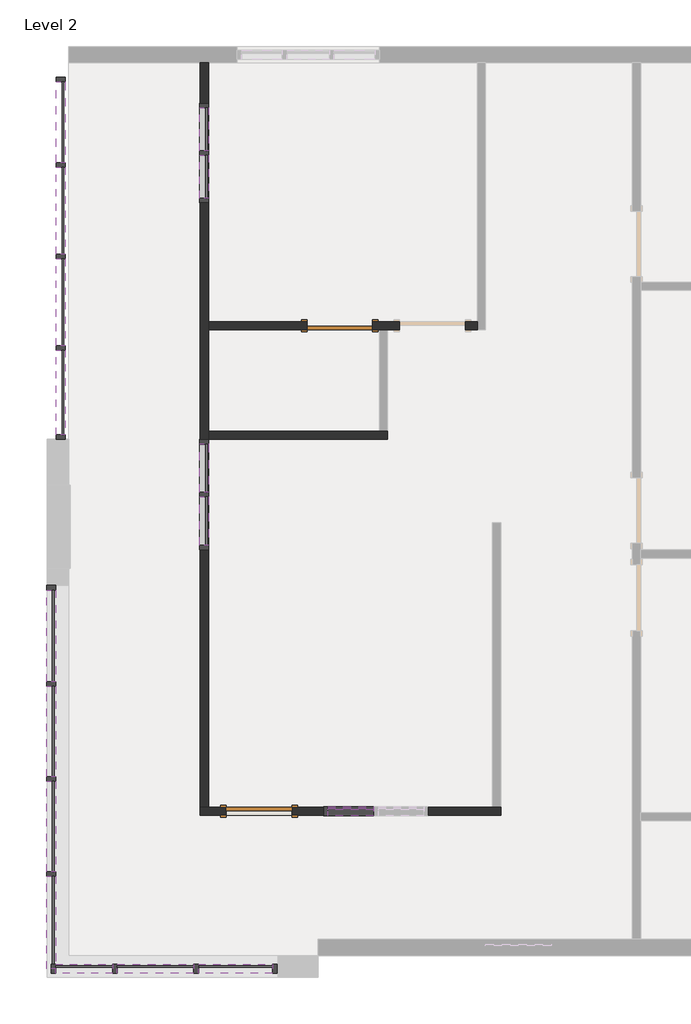
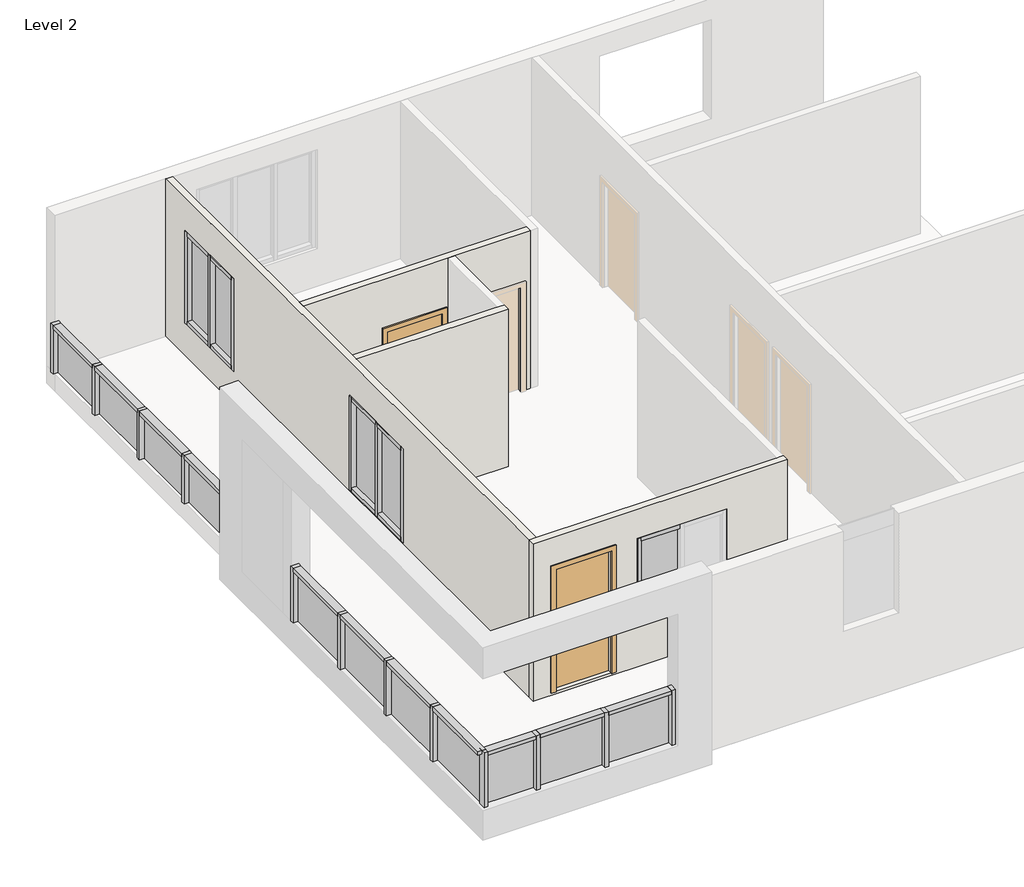
# One storey, part 1 of 2: 41 members, 16 plates, 4 walls, 2 doors.
"""IFC4 building model written with IfcOpenShell, lengths in millimetres."""

from ifc_helpers import new_model, si_unit, origin, place, context, project, spatial, faceted_brep, transform, mapped, element, save
from components import door_305aa2a5, member_a400357f, member_bc7c5251, member_6d802792, member_051277f3, member_fa50fb7e, member_1e79e512, member_04adda39, member_6ffa5180, member_e6b9f524, member_19f58c97, member_63803c1e, member_77473497, member_3cc93373, member_e1cb8a7d, member_bcb6a316, member_cba00588, member_798c2a08, member_45f34f4c, member_e49f56fc, member_c4de40ee, member_13dc6413, member_6ef8dc49, member_eb96f34d, system_panel_glazed_b36345c5, system_panel_glazed_219b4c74, system_panel_glazed_d508df5b, system_panel_glazed_98635403, system_panel_glazed_7a6fc0cf, system_panel_glazed_66c18ae2, system_panel_glazed_0daebeb7, system_panel_glazed_36a05233, system_panel_glazed_4373b602, system_panel_glazed_38c9bce4, system_panel_glazed_4a7c210e, system_panel_glazed_37b2116f

model = new_model("IFC4")

# Units and contexts
model_context = context("Model", 3, world=origin())
ifc_project = project(units=[si_unit("LENGTHUNIT", "METRE", prefix="MILLI")], contexts=[model_context])

# Site, building, storey
site = spatial("IfcSite", under=ifc_project)
building = spatial("IfcBuilding", under=site)
storey = spatial("IfcBuildingStorey", under=building, Name="Level 2", Elevation=3048.0)

# Doors
placement = place(None, origin())
door_shape = door_305aa2a5(model_context)
element("IfcDoor", 1, ObjectType="Single-Flush : 36\" x 84\"", at=placement, inside=storey, context=model_context, shape_type="MappedRepresentation", body=[
    mapped(door_shape, transform((-16492.8503587, -5110.3526331, 3048.0), x_axis=(1.0, 0.0, 0.0), y_axis=(0.0, 1.0, 0.0), z_axis=(0.0, 0.0, 1.0))),
])
element("IfcDoor", 2, ObjectType="Single-Flush : 36\" x 84\"", at=placement, inside=storey, context=model_context, shape_type="MappedRepresentation", body=[
    mapped(door_shape, transform((-17616.8003587, -11866.7526331, 3403.6), x_axis=(-1.0, 0.0, 0.0), y_axis=(0.0, -1.0, 0.0), z_axis=(0.0, 0.0, 1.0))),
])

# Members
member_shape = member_a400357f(model_context)
element("IfcMember", 3, ObjectType="Rectangular Mullion : 2.5\" x 5\" rectangular", at=placement, inside=storey, context=model_context, shape_type="MappedRepresentation", body=[
    mapped(member_shape, transform((-18378.8003587, -2671.9526331, 5536.2113847), x_axis=(0.0, 0.0, 1.0), y_axis=(-1.0, 0.0, 0.0), z_axis=(0.0, -1.0, 0.0))),
])
element("IfcMember", 4, ObjectType="Rectangular Mullion : 2.5\" x 5\" rectangular", at=placement, inside=storey, context=model_context, shape_type="MappedRepresentation", body=[
    mapped(member_shape, transform((-18378.8003587, -3332.3526331, 5536.2113847), x_axis=(0.0, 0.0, 1.0), y_axis=(-1.0, 0.0, 0.0), z_axis=(0.0, -1.0, 0.0))),
])
member_2_shape = member_bc7c5251(model_context)
element("IfcMember", 5, ObjectType="Rectangular Mullion : 2.5\" x 5\" rectangular", at=placement, inside=storey, context=model_context, shape_type="MappedRepresentation", body=[
    mapped(member_2_shape, transform((-18378.8003587, -2703.7026331, 3927.5904931), x_axis=(0.0, -1.0, 0.0), y_axis=(-1.0, 0.0, 0.0), z_axis=(0.0, 0.0, -1.0))),
])
element("IfcMember", 6, ObjectType="Rectangular Mullion : 2.5\" x 5\" rectangular", at=placement, inside=storey, context=model_context, shape_type="MappedRepresentation", body=[
    mapped(member_shape, transform((-18378.8003587, -2735.4526331, 3927.5904931), x_axis=(0.0, 0.0, -1.0), y_axis=(-1.0, 0.0, 0.0), z_axis=(0.0, 1.0, 0.0))),
])
element("IfcMember", 7, ObjectType="Rectangular Mullion : 2.5\" x 5\" rectangular", at=placement, inside=storey, context=model_context, shape_type="MappedRepresentation", body=[
    mapped(member_shape, transform((-18378.8003587, -2075.0526331, 3927.5904931), x_axis=(0.0, 0.0, -1.0), y_axis=(-1.0, 0.0, 0.0), z_axis=(0.0, 1.0, 0.0))),
])
member_3_shape = member_6d802792(model_context)
element("IfcMember", 8, ObjectType="Rectangular Mullion : 2.5\" x 5\" rectangular", at=placement, inside=storey, context=model_context, shape_type="MappedRepresentation", body=[
    mapped(member_3_shape, transform((-18378.8003587, -3395.8526331, 3927.5904931), x_axis=(0.0, -1.0, 0.0), y_axis=(-1.0, 0.0, 0.0), z_axis=(0.0, 0.0, -1.0))),
])
element("IfcMember", 9, ObjectType="Rectangular Mullion : 2.5\" x 5\" rectangular", at=placement, inside=storey, context=model_context, shape_type="MappedRepresentation", body=[
    mapped(member_3_shape, transform((-18378.8003587, -2011.5526331, 5536.2113847), x_axis=(0.0, 1.0, 0.0), y_axis=(-1.0, 0.0, 0.0), z_axis=(0.0, 0.0, 1.0))),
])
member_4_shape = member_051277f3(model_context)
element("IfcMember", 10, ObjectType="Rectangular Mullion : 2.5\" x 5\" rectangular", at=placement, inside=storey, context=model_context, shape_type="MappedRepresentation", body=[
    mapped(member_4_shape, transform((-18378.8003587, -7428.1026331, 5506.8936219), x_axis=(0.0, 0.0, 1.0), y_axis=(-1.0, 0.0, 0.0), z_axis=(0.0, -1.0, 0.0))),
])
element("IfcMember", 11, ObjectType="Rectangular Mullion : 2.5\" x 5\" rectangular", at=placement, inside=storey, context=model_context, shape_type="MappedRepresentation", body=[
    mapped(member_4_shape, transform((-18378.8003587, -8164.7026331, 5506.8936219), x_axis=(0.0, 0.0, 1.0), y_axis=(-1.0, 0.0, 0.0), z_axis=(0.0, -1.0, 0.0))),
])
member_5_shape = member_fa50fb7e(model_context)
element("IfcMember", 12, ObjectType="Rectangular Mullion : 2.5\" x 5\" rectangular", at=placement, inside=storey, context=model_context, shape_type="MappedRepresentation", body=[
    mapped(member_5_shape, transform((-18378.8003587, -7459.8526331, 3873.1435835), x_axis=(0.0, -1.0, 0.0), y_axis=(-1.0, 0.0, 0.0), z_axis=(0.0, 0.0, -1.0))),
])
element("IfcMember", 13, ObjectType="Rectangular Mullion : 2.5\" x 5\" rectangular", at=placement, inside=storey, context=model_context, shape_type="MappedRepresentation", body=[
    mapped(member_4_shape, transform((-18378.8003587, -7491.6026331, 3873.1435835), x_axis=(0.0, 0.0, -1.0), y_axis=(-1.0, 0.0, 0.0), z_axis=(0.0, 1.0, 0.0))),
])
element("IfcMember", 14, ObjectType="Rectangular Mullion : 2.5\" x 5\" rectangular", at=placement, inside=storey, context=model_context, shape_type="MappedRepresentation", body=[
    mapped(member_4_shape, transform((-18378.8003587, -6755.0026331, 3873.1435835), x_axis=(0.0, 0.0, -1.0), y_axis=(-1.0, 0.0, 0.0), z_axis=(0.0, 1.0, 0.0))),
])
member_6_shape = member_1e79e512(model_context)
element("IfcMember", 15, ObjectType="Rectangular Mullion : 2.5\" x 5\" rectangular", at=placement, inside=storey, context=model_context, shape_type="MappedRepresentation", body=[
    mapped(member_6_shape, transform((-18378.8003587, -6691.5026331, 5506.8936219), x_axis=(0.0, 1.0, 0.0), y_axis=(-1.0, 0.0, 0.0), z_axis=(0.0, 0.0, 1.0))),
])
element("IfcMember", 16, ObjectType="Rectangular Mullion : 2.5\" x 5\" rectangular", at=placement, inside=storey, context=model_context, shape_type="MappedRepresentation", body=[
    mapped(member_6_shape, transform((-18378.8003587, -8228.2026331, 3873.1435835), x_axis=(0.0, -1.0, 0.0), y_axis=(-1.0, 0.0, 0.0), z_axis=(0.0, 0.0, -1.0))),
])
member_7_shape = member_04adda39(model_context)
element("IfcMember", 17, ObjectType="Rectangular Mullion : 2.5\" x 5\" rectangular", at=placement, inside=storey, context=model_context, shape_type="MappedRepresentation", body=[
    mapped(member_7_shape, transform((-16019.7753587, -11866.7526331, 5586.8732654), x_axis=(0.0, 0.0, 1.0), y_axis=(0.0, -1.0, 0.0), z_axis=(1.0, 0.0, 0.0))),
])
element("IfcMember", 18, ObjectType="Rectangular Mullion : 2.5\" x 5\" rectangular", at=placement, inside=storey, context=model_context, shape_type="MappedRepresentation", body=[
    mapped(member_7_shape, transform((-16657.9503587, -11866.7526331, 4227.0998045), x_axis=(0.0, 0.0, -1.0), y_axis=(0.0, -1.0, 0.0), z_axis=(-1.0, 0.0, 0.0))),
])
member_8_shape = member_6ffa5180(model_context)
element("IfcMember", 19, ObjectType="Rectangular Mullion : 2.5\" x 5\" rectangular", at=placement, inside=storey, context=model_context, shape_type="MappedRepresentation", body=[
    mapped(member_8_shape, transform((-16721.4503587, -11866.7526331, 5586.8732654), x_axis=(-1.0, 0.0, 0.0), y_axis=(0.0, -1.0, 0.0), z_axis=(0.0, 0.0, 1.0))),
])
member_9_shape = member_e6b9f524(model_context)
element("IfcMember", 20, ObjectType="Rectangular Mullion : 2.5\" x 5\" rectangular", at=placement, inside=storey, context=model_context, shape_type="MappedRepresentation", body=[
    mapped(member_9_shape, transform((-20379.0503587, -2841.0830211, 4408.9968859), x_axis=(0.0, 0.0, 1.0), y_axis=(-1.0, 0.0, 0.0), z_axis=(0.0, -1.0, 0.0))),
])
member_10_shape = member_19f58c97(model_context)
element("IfcMember", 21, ObjectType="Rectangular Mullion : 2.5\" x 5\" rectangular", at=placement, inside=storey, context=model_context, shape_type="MappedRepresentation", body=[
    mapped(member_10_shape, transform((-20379.0503587, -1653.6330211, 4408.9968859), x_axis=(0.0, 1.0, 0.0), y_axis=(-1.0, 0.0, 0.0), z_axis=(0.0, 0.0, 1.0))),
])
member_11_shape = member_63803c1e(model_context)
element("IfcMember", 22, ObjectType="Rectangular Mullion : 2.5\" x 5\" rectangular", at=placement, inside=storey, context=model_context, shape_type="MappedRepresentation", body=[
    mapped(member_11_shape, transform((-20379.0503587, -2872.8330211, 3560.986402), x_axis=(0.0, -1.0, 0.0), y_axis=(-1.0, 0.0, 0.0), z_axis=(0.0, 0.0, -1.0))),
])
element("IfcMember", 23, ObjectType="Rectangular Mullion : 2.5\" x 5\" rectangular", at=placement, inside=storey, context=model_context, shape_type="MappedRepresentation", body=[
    mapped(member_11_shape, transform((-20379.0503587, -4145.7228918, 3560.986402), x_axis=(0.0, -1.0, 0.0), y_axis=(-1.0, 0.0, 0.0), z_axis=(0.0, 0.0, -1.0))),
])
element("IfcMember", 24, ObjectType="Rectangular Mullion : 2.5\" x 5\" rectangular", at=placement, inside=storey, context=model_context, shape_type="MappedRepresentation", body=[
    mapped(member_11_shape, transform((-20379.0503587, -5418.6127624, 3560.986402), x_axis=(0.0, -1.0, 0.0), y_axis=(-1.0, 0.0, 0.0), z_axis=(0.0, 0.0, -1.0))),
])
member_12_shape = member_77473497(model_context)
element("IfcMember", 25, ObjectType="Rectangular Mullion : 2.5\" x 5\" rectangular", at=placement, inside=storey, context=model_context, shape_type="MappedRepresentation", body=[
    mapped(member_12_shape, transform((-20379.0503587, -5386.8627624, 4408.9968859), x_axis=(0.0, 0.0, 1.0), y_axis=(-1.0, 0.0, 0.0), z_axis=(0.0, -1.0, 0.0))),
])
element("IfcMember", 26, ObjectType="Rectangular Mullion : 2.5\" x 5\" rectangular", at=placement, inside=storey, context=model_context, shape_type="MappedRepresentation", body=[
    mapped(member_12_shape, transform((-20379.0503587, -4113.9728918, 4408.9968859), x_axis=(0.0, 0.0, 1.0), y_axis=(-1.0, 0.0, 0.0), z_axis=(0.0, -1.0, 0.0))),
])
member_13_shape = member_3cc93373(model_context)
element("IfcMember", 27, ObjectType="Rectangular Mullion : 2.5\" x 5\" rectangular", at=placement, inside=storey, context=model_context, shape_type="MappedRepresentation", body=[
    mapped(member_13_shape, transform((-20379.0503587, -6628.0026331, 4408.9968859), x_axis=(0.0, 0.0, 1.0), y_axis=(-1.0, 0.0, 0.0), z_axis=(0.0, -1.0, 0.0))),
])
element("IfcMember", 28, ObjectType="Rectangular Mullion : 2.5\" x 5\" rectangular", at=placement, inside=storey, context=model_context, shape_type="MappedRepresentation", body=[
    mapped(member_10_shape, transform((-20379.0503587, -6691.5026331, 3560.986402), x_axis=(0.0, -1.0, 0.0), y_axis=(-1.0, 0.0, 0.0), z_axis=(0.0, 0.0, -1.0))),
])
member_14_shape = member_e1cb8a7d(model_context)
element("IfcMember", 29, ObjectType="Rectangular Mullion : 2.5\" x 5\" rectangular", at=placement, inside=storey, context=model_context, shape_type="MappedRepresentation", body=[
    mapped(member_14_shape, transform((-20512.4003587, -10095.1026331, 3560.986402), x_axis=(0.0, -1.0, 0.0), y_axis=(-1.0, 0.0, 0.0), z_axis=(0.0, 0.0, -1.0))),
])
element("IfcMember", 30, ObjectType="Rectangular Mullion : 2.5\" x 5\" rectangular", at=placement, inside=storey, context=model_context, shape_type="MappedRepresentation", body=[
    mapped(member_14_shape, transform((-20512.4003587, -11415.9026331, 3560.986402), x_axis=(0.0, -1.0, 0.0), y_axis=(-1.0, 0.0, 0.0), z_axis=(0.0, 0.0, -1.0))),
])
element("IfcMember", 31, ObjectType="Rectangular Mullion : 2.5\" x 5\" rectangular", at=placement, inside=storey, context=model_context, shape_type="MappedRepresentation", body=[
    mapped(member_14_shape, transform((-20512.4003587, -12736.7026331, 3560.986402), x_axis=(0.0, -1.0, 0.0), y_axis=(-1.0, 0.0, 0.0), z_axis=(0.0, 0.0, -1.0))),
])
member_15_shape = member_bcb6a316(model_context)
element("IfcMember", 32, ObjectType="Rectangular Mullion : 2.5\" x 5\" rectangular", at=placement, inside=storey, context=model_context, shape_type="MappedRepresentation", body=[
    mapped(member_15_shape, transform((-20512.4003587, -12704.9526331, 4515.4150439), x_axis=(0.0, 0.0, 1.0), y_axis=(-1.0, 0.0, 0.0), z_axis=(0.0, -1.0, 0.0))),
])
element("IfcMember", 33, ObjectType="Rectangular Mullion : 2.5\" x 5\" rectangular", at=placement, inside=storey, context=model_context, shape_type="MappedRepresentation", body=[
    mapped(member_15_shape, transform((-20512.4003587, -11384.1526331, 4515.4150439), x_axis=(0.0, 0.0, 1.0), y_axis=(-1.0, 0.0, 0.0), z_axis=(0.0, -1.0, 0.0))),
])
member_16_shape = member_cba00588(model_context)
element("IfcMember", 34, ObjectType="Rectangular Mullion : 2.5\" x 5\" rectangular", at=placement, inside=storey, context=model_context, shape_type="MappedRepresentation", body=[
    mapped(member_16_shape, transform((-20512.4003587, -10063.3526331, 4515.4150439), x_axis=(0.0, 0.0, 1.0), y_axis=(-1.0, 0.0, 0.0), z_axis=(0.0, -1.0, 0.0))),
])
member_17_shape = member_798c2a08(model_context)
element("IfcMember", 35, ObjectType="Rectangular Mullion : 2.5\" x 5\" rectangular", at=placement, inside=storey, context=model_context, shape_type="MappedRepresentation", body=[
    mapped(member_17_shape, transform((-20512.4003587, -14057.5026331, 4515.4150439), x_axis=(0.0, 0.0, 1.0), y_axis=(-1.0, 0.0, 0.0), z_axis=(0.0, -1.0, 0.0))),
])
member_18_shape = member_45f34f4c(model_context)
element("IfcMember", 36, ObjectType="Rectangular Mullion : 2.5\" x 5\" rectangular", at=placement, inside=storey, context=model_context, shape_type="MappedRepresentation", body=[
    mapped(member_18_shape, transform((-20512.4003587, -8723.5026331, 4515.4150439), x_axis=(0.0, 1.0, 0.0), y_axis=(-1.0, 0.0, 0.0), z_axis=(0.0, 0.0, 1.0))),
])
member_19_shape = member_e49f56fc(model_context)
element("IfcMember", 37, ObjectType="Rectangular Mullion : 2.5\" x 5\" rectangular", at=placement, inside=storey, context=model_context, shape_type="MappedRepresentation", body=[
    mapped(member_19_shape, transform((-19623.4003587, -14057.5026331, 3560.986402), x_axis=(1.0, 0.0, 0.0), y_axis=(0.0, -1.0, 0.0), z_axis=(0.0, 0.0, -1.0))),
])
element("IfcMember", 38, ObjectType="Rectangular Mullion : 2.5\" x 5\" rectangular", at=placement, inside=storey, context=model_context, shape_type="MappedRepresentation", body=[
    mapped(member_19_shape, transform((-18493.1003587, -14057.5026331, 3560.986402), x_axis=(1.0, 0.0, 0.0), y_axis=(0.0, -1.0, 0.0), z_axis=(0.0, 0.0, -1.0))),
])
member_20_shape = member_c4de40ee(model_context)
element("IfcMember", 39, ObjectType="Rectangular Mullion : 2.5\" x 5\" rectangular", at=placement, inside=storey, context=model_context, shape_type="MappedRepresentation", body=[
    mapped(member_20_shape, transform((-18524.8503587, -14057.5026331, 4515.0022133), x_axis=(0.0, 0.0, 1.0), y_axis=(0.0, -1.0, 0.0), z_axis=(1.0, 0.0, 0.0))),
])
member_21_shape = member_13dc6413(model_context)
element("IfcMember", 40, ObjectType="Rectangular Mullion : 2.5\" x 5\" rectangular", at=placement, inside=storey, context=model_context, shape_type="MappedRepresentation", body=[
    mapped(member_21_shape, transform((-19655.1503587, -14057.5026331, 4515.0022133), x_axis=(0.0, 0.0, 1.0), y_axis=(0.0, -1.0, 0.0), z_axis=(1.0, 0.0, 0.0))),
])
member_22_shape = member_6ef8dc49(model_context)
element("IfcMember", 41, ObjectType="Rectangular Mullion : 2.5\" x 5\" rectangular", at=placement, inside=storey, context=model_context, shape_type="MappedRepresentation", body=[
    mapped(member_22_shape, transform((-17426.3003587, -14057.5026331, 4515.0022133), x_axis=(0.0, 0.0, 1.0), y_axis=(0.0, -1.0, 0.0), z_axis=(1.0, 0.0, 0.0))),
])
member_23_shape = member_eb96f34d(model_context)
element("IfcMember", 42, ObjectType="Rectangular Mullion : 2.5\" x 5\" rectangular", at=placement, inside=storey, context=model_context, shape_type="MappedRepresentation", body=[
    mapped(member_23_shape, transform((-20512.4003587, -14057.5026331, 4515.0022133), x_axis=(-1.0, 0.0, 0.0), y_axis=(0.0, -1.0, 0.0), z_axis=(0.0, 0.0, 1.0))),
])
element("IfcMember", 43, ObjectType="Rectangular Mullion : 2.5\" x 5\" rectangular", at=placement, inside=storey, context=model_context, shape_type="MappedRepresentation", body=[
    mapped(member_23_shape, transform((-17362.8003587, -14057.5026331, 3560.986402), x_axis=(1.0, 0.0, 0.0), y_axis=(0.0, -1.0, 0.0), z_axis=(0.0, 0.0, -1.0))),
])

# Plates
system_panel_glazed_shape = system_panel_glazed_b36345c5(model_context)
element("IfcPlate", 44, ObjectType="System Panel : Glazed", at=placement, inside=storey, context=model_context, shape_type="MappedRepresentation", body=[
    mapped(system_panel_glazed_shape, transform((-18378.8003587, -2373.5026331, 3991.0904931), x_axis=(0.0, -1.0, 0.0), y_axis=(1.0, 0.0, 0.0), z_axis=(0.0, 0.0, 1.0))),
])
element("IfcPlate", 45, ObjectType="System Panel : Glazed", at=placement, inside=storey, context=model_context, shape_type="MappedRepresentation", body=[
    mapped(system_panel_glazed_shape, transform((-18378.8003587, -3033.9026331, 3991.0904931), x_axis=(0.0, -1.0, 0.0), y_axis=(1.0, 0.0, 0.0), z_axis=(0.0, 0.0, 1.0))),
])
system_panel_glazed_2_shape = system_panel_glazed_219b4c74(model_context)
element("IfcPlate", 46, ObjectType="System Panel : Glazed", at=placement, inside=storey, context=model_context, shape_type="MappedRepresentation", body=[
    mapped(system_panel_glazed_2_shape, transform((-18378.8003587, -7091.5526331, 3936.6435835), x_axis=(0.0, -1.0, 0.0), y_axis=(1.0, 0.0, 0.0), z_axis=(0.0, 0.0, 1.0))),
])
element("IfcPlate", 47, ObjectType="System Panel : Glazed", at=placement, inside=storey, context=model_context, shape_type="MappedRepresentation", body=[
    mapped(system_panel_glazed_2_shape, transform((-18378.8003587, -7828.1526331, 3936.6435835), x_axis=(0.0, -1.0, 0.0), y_axis=(1.0, 0.0, 0.0), z_axis=(0.0, 0.0, 1.0))),
])
system_panel_glazed_3_shape = system_panel_glazed_d508df5b(model_context)
element("IfcPlate", 48, ObjectType="System Panel : Glazed", at=placement, inside=storey, context=model_context, shape_type="MappedRepresentation", body=[
    mapped(system_panel_glazed_3_shape, transform((-16338.8628587, -11866.7526331, 4290.5998045), x_axis=(1.0, 0.0, 0.0), y_axis=(0.0, 1.0, 0.0), z_axis=(0.0, 0.0, 1.0))),
])
system_panel_glazed_4_shape = system_panel_glazed_98635403(model_context)
element("IfcPlate", 49, ObjectType="System Panel : Glazed", at=placement, inside=storey, context=model_context, shape_type="MappedRepresentation", body=[
    mapped(system_panel_glazed_4_shape, transform((-20379.0503587, -2279.1080211, 3560.986402), x_axis=(0.0, -1.0, 0.0), y_axis=(1.0, 0.0, 0.0), z_axis=(0.0, 0.0, 1.0))),
])
system_panel_glazed_5_shape = system_panel_glazed_7a6fc0cf(model_context)
element("IfcPlate", 50, ObjectType="System Panel : Glazed", at=placement, inside=storey, context=model_context, shape_type="MappedRepresentation", body=[
    mapped(system_panel_glazed_5_shape, transform((-20379.0503587, -3509.2779565, 3560.986402), x_axis=(0.0, -1.0, 0.0), y_axis=(1.0, 0.0, 0.0), z_axis=(0.0, 0.0, 1.0))),
])
element("IfcPlate", 51, ObjectType="System Panel : Glazed", at=placement, inside=storey, context=model_context, shape_type="MappedRepresentation", body=[
    mapped(system_panel_glazed_5_shape, transform((-20379.0503587, -4782.1678271, 3560.986402), x_axis=(0.0, -1.0, 0.0), y_axis=(1.0, 0.0, 0.0), z_axis=(0.0, 0.0, 1.0))),
])
system_panel_glazed_6_shape = system_panel_glazed_66c18ae2(model_context)
element("IfcPlate", 52, ObjectType="System Panel : Glazed", at=placement, inside=storey, context=model_context, shape_type="MappedRepresentation", body=[
    mapped(system_panel_glazed_6_shape, transform((-20379.0503587, -6039.1826978, 3560.986402), x_axis=(0.0, -1.0, 0.0), y_axis=(1.0, 0.0, 0.0), z_axis=(0.0, 0.0, 1.0))),
])
system_panel_glazed_7_shape = system_panel_glazed_0daebeb7(model_context)
element("IfcPlate", 53, ObjectType="System Panel : Glazed", at=placement, inside=storey, context=model_context, shape_type="MappedRepresentation", body=[
    mapped(system_panel_glazed_7_shape, transform((-20512.4003587, -9425.1776331, 3560.986402), x_axis=(0.0, -1.0, 0.0), y_axis=(1.0, 0.0, 0.0), z_axis=(0.0, 0.0, 1.0))),
])
system_panel_glazed_8_shape = system_panel_glazed_36a05233(model_context)
element("IfcPlate", 54, ObjectType="System Panel : Glazed", at=placement, inside=storey, context=model_context, shape_type="MappedRepresentation", body=[
    mapped(system_panel_glazed_8_shape, transform((-20512.4003587, -10755.5026331, 3560.986402), x_axis=(0.0, -1.0, 0.0), y_axis=(1.0, 0.0, 0.0), z_axis=(0.0, 0.0, 1.0))),
])
element("IfcPlate", 55, ObjectType="System Panel : Glazed", at=placement, inside=storey, context=model_context, shape_type="MappedRepresentation", body=[
    mapped(system_panel_glazed_8_shape, transform((-20512.4003587, -12076.3026331, 3560.986402), x_axis=(0.0, -1.0, 0.0), y_axis=(1.0, 0.0, 0.0), z_axis=(0.0, 0.0, 1.0))),
])
system_panel_glazed_9_shape = system_panel_glazed_4373b602(model_context)
element("IfcPlate", 56, ObjectType="System Panel : Glazed", at=placement, inside=storey, context=model_context, shape_type="MappedRepresentation", body=[
    mapped(system_panel_glazed_9_shape, transform((-20512.4003587, -13412.9776331, 3560.986402), x_axis=(0.0, -1.0, 0.0), y_axis=(1.0, 0.0, 0.0), z_axis=(0.0, 0.0, 1.0))),
])
system_panel_glazed_10_shape = system_panel_glazed_38c9bce4(model_context)
element("IfcPlate", 57, ObjectType="System Panel : Glazed", at=placement, inside=storey, context=model_context, shape_type="MappedRepresentation", body=[
    mapped(system_panel_glazed_10_shape, transform((-20052.0253587, -14057.5026331, 3560.986402), x_axis=(1.0, 0.0, 0.0), y_axis=(0.0, 1.0, 0.0), z_axis=(0.0, 0.0, 1.0))),
])
system_panel_glazed_11_shape = system_panel_glazed_4a7c210e(model_context)
element("IfcPlate", 58, ObjectType="System Panel : Glazed", at=placement, inside=storey, context=model_context, shape_type="MappedRepresentation", body=[
    mapped(system_panel_glazed_11_shape, transform((-19058.2503587, -14057.5026331, 3560.986402), x_axis=(1.0, 0.0, 0.0), y_axis=(0.0, 1.0, 0.0), z_axis=(0.0, 0.0, 1.0))),
])
system_panel_glazed_12_shape = system_panel_glazed_37b2116f(model_context)
element("IfcPlate", 59, ObjectType="System Panel : Glazed", at=placement, inside=storey, context=model_context, shape_type="MappedRepresentation", body=[
    mapped(system_panel_glazed_12_shape, transform((-17943.8253587, -14057.5026331, 3560.986402), x_axis=(1.0, 0.0, 0.0), y_axis=(0.0, 1.0, 0.0), z_axis=(0.0, 0.0, 1.0))),
])

# Walls
element("IfcWall", 60, ObjectType="4.5\"", at=placement, inside=storey, context=model_context, shape_type="Brep", body=[
    faceted_brep([(-18435.9503587, -1452.7526331, 3048.0), (-18435.9503587, -11809.6026331, 3048.0), (-18435.9503587, -11809.6026331, 6096.0), (-18435.9503587, -1452.7526331, 6096.0), (-18435.9503587, -2011.5526331, 3927.5904931), (-18435.9503587, -2011.5526331, 5536.2113847), (-18435.9503587, -3395.8526331, 5536.2113847), (-18435.9503587, -3395.8526331, 3927.5904931), (-18435.9503587, -6691.5026331, 3873.1435835), (-18435.9503587, -6691.5026331, 5506.8936219), (-18435.9503587, -8228.2026331, 5506.8936219), (-18435.9503587, -8228.2026331, 3873.1435835), (-18321.6503587, -11809.6026331, 3048.0), (-18321.6503587, -6691.5026331, 3048.0), (-18321.6503587, -6577.2026331, 3048.0), (-18321.6503587, -5167.5026331, 3048.0), (-18321.6503587, -5053.2026331, 3048.0), (-18321.6503587, -1452.7526331, 3048.0), (-18321.6503587, -1452.7526331, 6096.0), (-18321.6503587, -5053.2026331, 6096.0), (-18321.6503587, -5167.5026331, 6096.0), (-18321.6503587, -6577.2026331, 6096.0), (-18321.6503587, -6691.5026331, 6096.0), (-18321.6503587, -11809.6026331, 6096.0), (-18321.6503587, -2011.5526331, 5536.2113847), (-18321.6503587, -2011.5526331, 3927.5904931), (-18321.6503587, -3395.8526331, 3927.5904931), (-18321.6503587, -3395.8526331, 5536.2113847), (-18321.6503587, -6691.5026331, 5506.8936219), (-18321.6503587, -6691.5026331, 3873.1435835), (-18321.6503587, -8228.2026331, 3873.1435835), (-18321.6503587, -8228.2026331, 5506.8936219)], [[[0, 1, 2, 3], [4, 5, 6, 7], [8, 9, 10, 11]], [[12, 13, 14, 15, 16, 17, 18, 19, 20, 21, 22, 23], [24, 25, 26, 27], [28, 29, 30, 31]], [[0, 3, 18, 17]], [[2, 1, 12, 23]], [[4, 25, 24, 5]], [[5, 24, 27, 6]], [[6, 27, 26, 7]], [[25, 4, 7, 26]], [[8, 29, 28, 9]], [[9, 28, 31, 10]], [[30, 11, 10, 31]], [[29, 8, 11, 30]], [[1, 0, 17, 16, 15, 14, 13, 12]], [[3, 2, 23, 22, 21, 20, 19, 18]]]),
])
element("IfcWall", 61, ObjectType="4.5\"", at=placement, inside=storey, context=model_context, shape_type="Brep", body=[
    faceted_brep([(-15657.8253587, -5053.2026331, 3048.0), (-16035.6503587, -5053.2026331, 3048.0), (-16035.6503587, -5053.2026331, 5181.6), (-16950.0503587, -5053.2026331, 5181.6), (-16950.0503587, -5053.2026331, 3048.0), (-18321.6503587, -5053.2026331, 3048.0), (-18321.6503587, -5053.2026331, 6096.0), (-14575.1503587, -5053.2026331, 6096.0), (-14575.1503587, -5053.2026331, 3048.0), (-14743.4253587, -5053.2026331, 3048.0), (-14743.4253587, -5053.2026331, 5181.6), (-15657.8253587, -5053.2026331, 5181.6), (-16035.6503587, -5167.5026331, 5181.6), (-16035.6503587, -5167.5026331, 3048.0), (-15940.4003587, -5167.5026331, 3048.0), (-15826.1003587, -5167.5026331, 3048.0), (-15657.8253587, -5167.5026331, 3048.0), (-15657.8253587, -5167.5026331, 5181.6), (-14743.4253587, -5167.5026331, 5181.6), (-14743.4253587, -5167.5026331, 3048.0), (-14575.1503587, -5167.5026331, 3048.0), (-14575.1503587, -5167.5026331, 6096.0), (-15826.1003587, -5167.5026331, 6096.0), (-15940.4003587, -5167.5026331, 6096.0), (-18321.6503587, -5167.5026331, 6096.0), (-18321.6503587, -5167.5026331, 3048.0), (-16950.0503587, -5167.5026331, 3048.0), (-16950.0503587, -5167.5026331, 5181.6)], [[[0, 1, 2, 3, 4, 5, 6, 7, 8, 9, 10, 11]], [[12, 13, 14, 15, 16, 17, 18, 19, 20, 21, 22, 23, 24, 25, 26, 27]], [[20, 19, 9, 8]], [[26, 25, 5, 4]], [[16, 15, 14, 13, 1, 0]], [[7, 6, 24, 23, 22, 21]], [[8, 7, 21, 20]], [[6, 5, 25, 24]], [[10, 9, 19, 18]], [[11, 10, 18, 17]], [[0, 11, 17, 16]], [[2, 1, 13, 12]], [[3, 2, 12, 27]], [[4, 3, 27, 26]]]),
])
element("IfcWall", 62, ObjectType="4.5\"", at=placement, inside=storey, context=model_context, shape_type="Brep", body=[
    faceted_brep([(-18321.6503587, -6691.5026331, 3048.0), (-15826.1003587, -6691.5026331, 3048.0), (-15826.1003587, -6691.5026331, 6096.0), (-18321.6503587, -6691.5026331, 6096.0), (-18321.6503587, -6691.5026331, 5506.8936219), (-18321.6503587, -6691.5026331, 3873.1435835), (-18321.6503587, -6577.2026331, 3048.0), (-18321.6503587, -6577.2026331, 6096.0), (-15940.4003587, -6577.2026331, 6096.0), (-15826.1003587, -6577.2026331, 6096.0), (-15826.1003587, -6577.2026331, 3048.0), (-15940.4003587, -6577.2026331, 3048.0)], [[[0, 1, 2, 3, 4, 5]], [[6, 7, 8, 9, 10, 11]], [[1, 0, 6, 11, 10]], [[3, 2, 9, 8, 7]], [[0, 5, 4, 3, 7, 6]], [[2, 1, 10, 9]]]),
])
element("IfcWall", 63, ObjectType="4.5\"", at=placement, inside=storey, context=model_context, shape_type="Brep", body=[
    faceted_brep([(-18435.9503587, -11923.9026331, 3048.0), (-14251.3003587, -11923.9026331, 3048.0), (-14251.3003587, -11923.9026331, 6096.0), (-18435.9503587, -11923.9026331, 6096.0), (-17159.6003587, -11923.9026331, 3403.6), (-18074.0003587, -11923.9026331, 3403.6), (-18074.0003587, -11923.9026331, 5537.2), (-17159.6003587, -11923.9026331, 5537.2), (-16721.4503587, -11923.9026331, 4227.0998045), (-16721.4503587, -11923.9026331, 5586.8732654), (-15254.6003587, -11923.9026331, 5586.8732654), (-15254.6003587, -11923.9026331, 4227.0998045), (-14251.3003587, -11809.6026331, 3048.0), (-14365.6003587, -11809.6026331, 3048.0), (-18321.6503587, -11809.6026331, 3048.0), (-18435.9503587, -11809.6026331, 3048.0), (-18435.9503587, -11809.6026331, 6096.0), (-18321.6503587, -11809.6026331, 6096.0), (-14365.6003587, -11809.6026331, 6096.0), (-14251.3003587, -11809.6026331, 6096.0), (-18074.0003587, -11809.6026331, 3403.6), (-17159.6003587, -11809.6026331, 3403.6), (-17159.6003587, -11809.6026331, 5537.2), (-18074.0003587, -11809.6026331, 5537.2), (-16721.4503587, -11809.6026331, 5586.8732654), (-16721.4503587, -11809.6026331, 4227.0998045), (-15254.6003587, -11809.6026331, 4227.0998045), (-15254.6003587, -11809.6026331, 5586.8732654)], [[[0, 1, 2, 3], [4, 5, 6, 7], [8, 9, 10, 11]], [[12, 13, 14, 15, 16, 17, 18, 19], [20, 21, 22, 23], [24, 25, 26, 27]], [[1, 0, 15, 14, 13, 12]], [[3, 2, 19, 18, 17, 16]], [[2, 1, 12, 19]], [[0, 3, 16, 15]], [[5, 4, 21, 20]], [[6, 5, 20, 23]], [[7, 6, 23, 22]], [[4, 7, 22, 21]], [[8, 25, 24, 9]], [[9, 24, 27, 10]], [[10, 27, 26, 11]], [[25, 8, 11, 26]]]),
])

save(model, "model.ifc")

# Revit data of these elements
# Type "Single-Flush : 36\" x 84\""
#   Type Mark = "1"
#   Construction Type Id = "MDOOR"
#   Assembly Code = "C1020"
#   Analytic Construction = "Metal"
#   Thickness = 0' - 2"
#   Heat Transfer Coefficient (U) = 0.651978 BTU/(h·ft²·°F)
#   Height = 7' - 0"
#   Trim Projection Ext = 0' - 1"
#   Trim Projection Int = 0' - 1"
#   Trim Width = 0' - 3"
#   Width = 3' - 0"
#   Define Thermal Properties by = 1
#   Define Thermal Properties by = 1
#   Door Material = Door - Panel
#   Frame Material = Door - Frame
#   Visual Light Transmittance = 0
#   Solar Heat Gain Coefficient = 0
#   Function = (empty or 0)
#   Wall Closure = (empty or 0)
# Type "Rectangular Mullion : 2.5\" x 5\" rectangular"
#   built-in parameter 1007304 = 0.416667 (stored number, unit not read)
#   built-in parameter 1007301 = 0.104167 (stored number, unit not read)
#   built-in parameter 1007300 = 0.104167 (stored number, unit not read)
# Type "System Panel : Glazed"
#   Construction Type Id = "GSP4R"
#   Analytic Construction = "1/8 in Pilkington single glazing"
#   Visual Light Transmittance = 0.9
#   Solar Heat Gain Coefficient = 0.86
#   Heat Transfer Coefficient (U) = 1.18115 BTU/(h·ft²·°F)
#   Define Thermal Properties by = 1
# Type "4.5\""
#   Assembly Code = "B2010"
#   Layers, outside or top first: 0' - 4 1/2" no material (function 1)
# Elements 1, 2 (IfcDoor, "Single-Flush : 36\" x 84\"")
#   Phase Created = New Construction
#   Materials on its faces: "Door - Frame", "Door - Panel"
# Elements 3, 4, 5, 6, 7, 8, 9, 10, 11, 12, 13, 14, 15, 16, 17, 18, 19, 20, 21, 22, 23, 24, 25, 26, 27, 28, 29, 30, 31, 32, 33, 34, 35, 36, 37, 38, 39, 40, 41, 42, 43 (IfcMember, "Rectangular Mullion : 2.5\" x 5\" rectangular")
#   Phase Created = New Construction
#   Materials on its faces: "Aluminum"
# Elements 44, 45, 46, 47, 48, 49, 50, 51, 52, 53, 54, 55, 56, 57, 58, 59 (IfcPlate, "System Panel : Glazed")
#   Phase Created = New Construction
#   Materials on its faces: "Glass"
# Elements 60, 61, 62, 63 (IfcWall, "4.5\"")
#   Top Offset = 0' - 0"
#   Base Offset = 0' - 0"
#   Unconnected Height = 10' - 0"
#   wall height = 10' - 0"
#   Phase Created = New Construction
#   Base Constraint = Level 2
#   Materials on its faces: "Default Wall"
# Materials
#   "Door - Panel": class "Wood", colour RGB 210 159 95, transparency 0, Cost = 0
#   "Door - Frame": colour RGB 118 70 51, transparency 0, Cost = 0
#   "Aluminum": class "Metal", colour RGB 247 247 247, transparency 0, Description = "Aluminum 6061", Cost = 0
#   "Glass": class "Glass", colour RGB 0 128 192, transparency 0.75, Description = "Soda Lime Glass", Cost = 0
#   "Default Wall": colour RGB 128 128 128, transparency 0, Cost = 0
